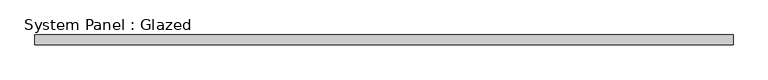
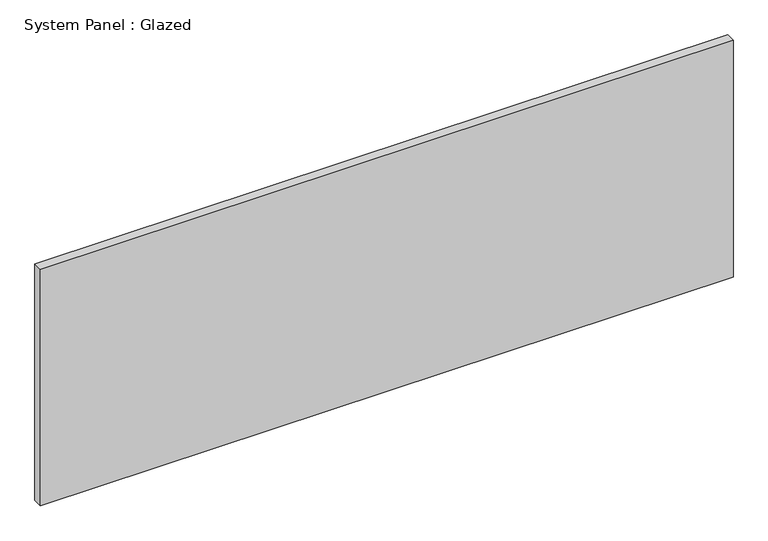
"""IFC4 building model written with IfcOpenShell, lengths in millimetres: plate geometry, System Panel : Glazed."""

from ifc_helpers import new_model, si_unit, origin, origin_with_axes, place, context, project, spatial, polyline, outline, extrude, source, transform, mapped, element, save


def system_panel_glazed_62d6a88c(model_context):
    return source(origin(), model_context, "Body", "SweptSolid", [
        extrude(outline(polyline([(914.4, 19.05), (-914.4, 19.05), (-914.4, 44.45), (914.4, 44.45), (914.4, 19.05)])), origin_with_axes(), (0.0, 0.0, 1.0), 660.4),
    ])


if __name__ == "__main__":
    model = new_model("IFC4")
    model_context = context("Model", 3, world=origin())
    ifc_project = project(units=[si_unit("LENGTHUNIT", "METRE", prefix="MILLI")], contexts=[model_context])
    site = spatial("IfcSite", under=ifc_project)
    building = spatial("IfcBuilding", under=site)
    placement = place(None, origin())
    system_panel_glazed_shape = system_panel_glazed_62d6a88c(model_context)
    element("IfcPlate", 1, ObjectType="System Panel : Glazed", at=placement, inside=building, context=model_context, shape_type="MappedRepresentation", body=[
        mapped(system_panel_glazed_shape, transform((0.0, 0.0, 0.0), x_axis=(1.0, 0.0, 0.0), y_axis=(0.0, 1.0, 0.0), z_axis=(0.0, 0.0, 1.0))),
    ])
    save(model, "model.ifc")

# Revit data of these elements
# Type "System Panel : Glazed"
#   Construction Type Id = "GSP4R"
#   Analytic Construction = "1/8 in Pilkington single glazing"
#   Visual Light Transmittance = 0.9
#   Solar Heat Gain Coefficient = 0.86
#   Heat Transfer Coefficient (U) = 1.18115 BTU/(h·ft²·°F)
# Element 1 (IfcPlate, "System Panel : Glazed")
#   Materials on its faces: "Glass"
# Materials
#   "Glass": class "Glass", colour RGB 0 128 192, transparency 0.75, Description = "Soda Lime Glass", Cost = 0
